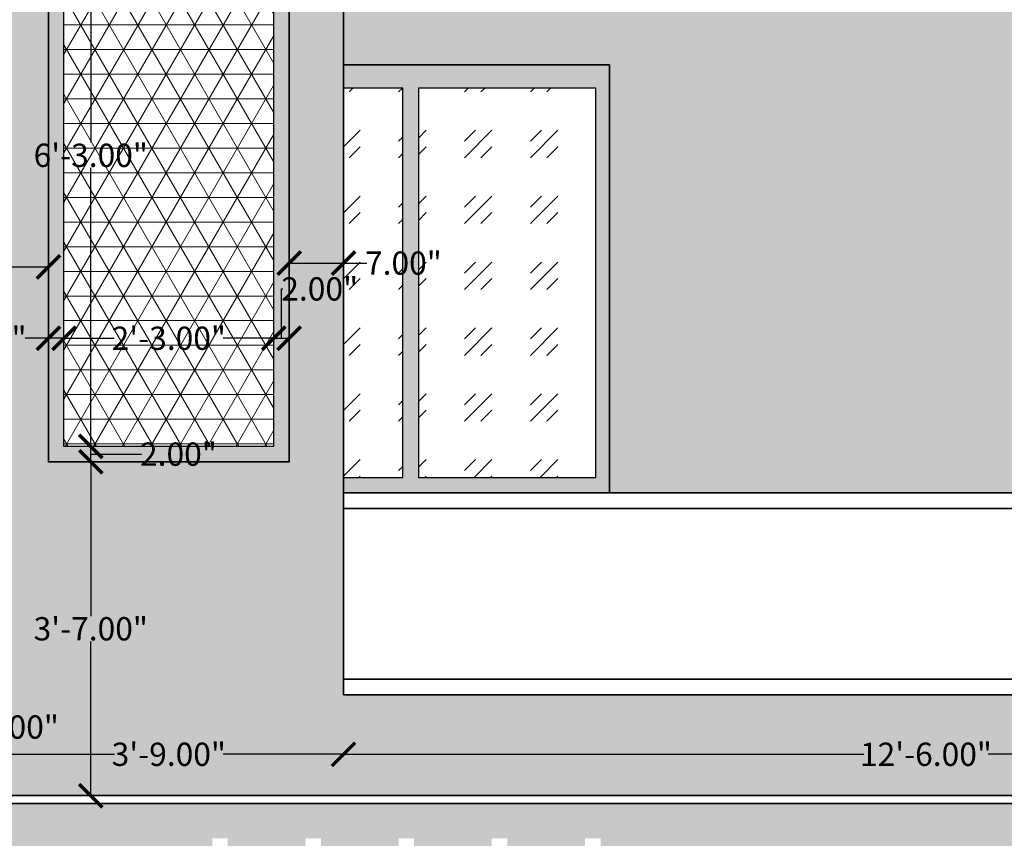
# Model space of a CAD drawing. Units: inches. Extents: x -654 to 390, y -40 to 648.
# Tile 7 of 13: x 104 to 231, y 311 to 417. Entities that reach past the tile are written whole.
import ezdxf

# ---------------------------------------------------------------- set-up
doc = ezdxf.new("R2010")
doc.units = ezdxf.units.IN
doc.header["$PDMODE"] = 3
for name, color, linetype, lineweight in [('A-ANNO-DIMS', 2, 'Continuous', 18), ('A-ELEV', 7, 'Continuous', 35), ('A-ELEV-FILL', 252, 'Continuous', 13), ('A-ELEV-PATT', 8, 'Continuous', 13), ('A-GLAZ', 4, 'Continuous', 25)]:
    doc.layers.add(name, color=color, linetype=linetype, lineweight=lineweight)
doc.styles.get("Standard").update_dxf_attribs({"font": 'arial.ttf'})
doc.dimstyles.get("Standard").update_dxf_attribs({"dimtxt": 3, "dimasz": 3, "dimexe": 0.18, "dimexo": 0.0625, "dimgap": 0.09, "dimtad": 0, "dimtih": 1, "dimtoh": 1, "dimzin": 0, "dimdsep": 46, "dimlunit": 3, "dimtxsty": 'Standard', "dimblk": 'ARCHTICK', "dimcen": 0.09, "dimse1": 1, "dimse2": 1, "dimadec": 0, "dimazin": 0, "dimtfac": 1, "dimtofl": 0, "dimtmove": 0, "dimatfit": 3, "dimfxl": 1, "dimtolj": 1, "dimtzin": 0, "dimarcsym": 0})

# ---------------------------------------------------------------- blocks, each defined once
blk = doc.blocks.new('_ArchTick')
at = {"color": 0, "linetype": 'ByBlock', "const_width": 0.15}
blk.add_lwpolyline([(-0.5, -0.5), (0.5, 0.5)], dxfattribs=at)
blk = doc.blocks.new('*D45')
at = {"layer": 'A-ANNO-DIMS', "color": 0, "lineweight": -2, "transparency": 16777216}
for p, q in [((99.15, 322.17), (99.15, 325.47)), ((99.15, 325.47), (99.33, 325.47)), ((100.65, 322.17), (97.65, 322.17))]:
    blk.add_line(p, q, dxfattribs=at)
at = {"layer": 'Defpoints', "color": 0, "transparency": 16777216}
for p in [(97.65, 322.17), (97.65, 316.63), (100.65, 316.63)]:
    blk.add_point(p, dxfattribs=at)
at = {"layer": 'A-ANNO-DIMS', "color": 0, "lineweight": -2, "transparency": 16777216, "xscale": 3, "yscale": 3, "zscale": 3, "rotation": 180}
blk.add_blockref('_ArchTick', (97.65, 322.17), dxfattribs=at)
at = {"layer": 'A-ANNO-DIMS', "color": 0, "lineweight": -2, "transparency": 16777216, "xscale": 3, "yscale": 3, "zscale": 3}
blk.add_blockref('_ArchTick', (100.65, 322.17), dxfattribs=at)
at = {"layer": 'A-ANNO-DIMS', "color": 0, "transparency": 16777216, "insert": (104.05, 325.47), "char_height": 3, "attachment_point": 5}
blk.add_mtext('\\A1;3.00"', dxfattribs=at)
blk = doc.blocks.new('*D46')
at = {"layer": 'A-ANNO-DIMS', "color": 0, "lineweight": -2, "transparency": 16777216}
for p, q in [((145.65, 321.96), (212.63, 321.96)), ((295.65, 321.96), (228.66, 321.96))]:
    blk.add_line(p, q, dxfattribs=at)
at = {"layer": 'Defpoints', "color": 0, "transparency": 16777216}
for p in [(145.65, 329.63), (145.65, 321.96), (295.65, 316.63)]:
    blk.add_point(p, dxfattribs=at)
at = {"layer": 'A-ANNO-DIMS', "color": 0, "lineweight": -2, "transparency": 16777216, "xscale": 3, "yscale": 3, "zscale": 3, "rotation": 180}
blk.add_blockref('_ArchTick', (145.65, 321.96), dxfattribs=at)
at = {"layer": 'A-ANNO-DIMS', "color": 0, "lineweight": -2, "transparency": 16777216, "xscale": 3, "yscale": 3, "zscale": 3}
blk.add_blockref('_ArchTick', (295.65, 321.96), dxfattribs=at)
at = {"layer": 'A-ANNO-DIMS', "color": 0, "transparency": 16777216, "insert": (220.65, 321.96), "char_height": 3, "attachment_point": 5}
blk.add_mtext('\\A1;12\'-6.00"', dxfattribs=at)
blk = doc.blocks.new('*D47')
at = {"layer": 'A-ANNO-DIMS', "color": 0, "lineweight": -2, "transparency": 16777216}
for p, q in [((100.65, 321.96), (116.16, 321.96)), ((145.65, 321.96), (130.14, 321.96))]:
    blk.add_line(p, q, dxfattribs=at)
at = {"layer": 'Defpoints', "color": 0, "transparency": 16777216}
for p in [(145.65, 329.63), (100.65, 322.17), (100.65, 321.96)]:
    blk.add_point(p, dxfattribs=at)
at = {"layer": 'A-ANNO-DIMS', "color": 0, "lineweight": -2, "transparency": 16777216, "xscale": 3, "yscale": 3, "zscale": 3, "rotation": 180}
blk.add_blockref('_ArchTick', (100.65, 321.96), dxfattribs=at)
at = {"layer": 'A-ANNO-DIMS', "color": 0, "lineweight": -2, "transparency": 16777216, "xscale": 3, "yscale": 3, "zscale": 3}
blk.add_blockref('_ArchTick', (145.65, 321.96), dxfattribs=at)
at = {"layer": 'A-ANNO-DIMS', "color": 0, "transparency": 16777216, "insert": (123.15, 321.96), "char_height": 3, "attachment_point": 5}
blk.add_mtext('\\A1;3\'-9.00"', dxfattribs=at)
blk = doc.blocks.new('*D48')
at = {"layer": 'A-ANNO-DIMS', "color": 0, "lineweight": -2, "transparency": 16777216}
for p, q in [((113.1, 359.63), (113.1, 339.76)), ((113.1, 316.63), (113.1, 336.51))]:
    blk.add_line(p, q, dxfattribs=at)
at = {"layer": 'Defpoints', "color": 0, "transparency": 16777216}
for p in [(107.65, 359.63), (113.1, 359.63), (100.65, 316.63)]:
    blk.add_point(p, dxfattribs=at)
at = {"layer": 'A-ANNO-DIMS', "color": 0, "lineweight": -2, "transparency": 16777216, "xscale": 3, "yscale": 3, "zscale": 3}
for p, rotation in [((113.1, 359.63), 90), ((113.1, 316.63), 270)]:
    blk.add_blockref('_ArchTick', p, dxfattribs=dict(at, rotation=rotation))
at = {"layer": 'A-ANNO-DIMS', "color": 0, "transparency": 16777216, "insert": (113.1, 338.13), "char_height": 3, "attachment_point": 5}
blk.add_mtext('\\A1;3\'-7.00"', dxfattribs=at)
blk = doc.blocks.new('*D49')
at = {"layer": 'A-ANNO-DIMS', "color": 0, "lineweight": -2, "transparency": 16777216}
for p, q in [((113.1, 359.63), (113.1, 361.63)), ((113.1, 360.63), (119.45, 360.63)), ((119.45, 360.63), (119.63, 360.63))]:
    blk.add_line(p, q, dxfattribs=at)
at = {"layer": 'Defpoints', "color": 0, "transparency": 16777216}
for p in [(113.1, 361.63), (113.1, 361.63), (107.65, 359.63)]:
    blk.add_point(p, dxfattribs=at)
at = {"layer": 'A-ANNO-DIMS', "color": 0, "lineweight": -2, "transparency": 16777216, "xscale": 3, "yscale": 3, "zscale": 3}
for p, rotation in [((113.1, 361.63), 90), ((113.1, 359.63), 270)]:
    blk.add_blockref('_ArchTick', p, dxfattribs=dict(at, rotation=rotation))
at = {"layer": 'A-ANNO-DIMS', "color": 0, "transparency": 16777216, "insert": (124.39, 360.63), "char_height": 3, "attachment_point": 5}
blk.add_mtext('\\A1;2.00"', dxfattribs=at)
blk = doc.blocks.new('*D50')
at = {"layer": 'A-ANNO-DIMS', "color": 0, "lineweight": -2, "transparency": 16777216}
for p, q in [((113.1, 436.63), (113.1, 400.76)), ((113.1, 361.63), (113.1, 397.51))]:
    blk.add_line(p, q, dxfattribs=at)
at = {"layer": 'Defpoints', "color": 0, "transparency": 16777216}
for p in [(113.1, 436.63), (113.1, 436.63), (113.1, 361.63)]:
    blk.add_point(p, dxfattribs=at)
at = {"layer": 'A-ANNO-DIMS', "color": 0, "lineweight": -2, "transparency": 16777216, "xscale": 3, "yscale": 3, "zscale": 3}
for p, rotation in [((113.1, 436.63), 90), ((113.1, 361.63), 270)]:
    blk.add_blockref('_ArchTick', p, dxfattribs=dict(at, rotation=rotation))
at = {"layer": 'A-ANNO-DIMS', "color": 0, "transparency": 16777216, "insert": (113.1, 399.13), "char_height": 3, "attachment_point": 5}
blk.add_mtext('\\A1;6\'-3.00"', dxfattribs=at)
blk = doc.blocks.new('*D53')
at = {"layer": 'A-ANNO-DIMS', "color": 0, "lineweight": -2, "transparency": 16777216}
for p, q in [((100.65, 384.74), (97.65, 384.74)), ((107.65, 384.74), (100.65, 384.74))]:
    blk.add_line(p, q, dxfattribs=at)
at = {"layer": 'Defpoints', "color": 0, "transparency": 16777216}
for p in [(100.65, 384.74), (100.65, 359.63), (107.65, 359.63)]:
    blk.add_point(p, dxfattribs=at)
at = {"layer": 'A-ANNO-DIMS', "color": 0, "lineweight": -2, "transparency": 16777216, "xscale": 3, "yscale": 3, "zscale": 3, "rotation": 180}
blk.add_blockref('_ArchTick', (100.65, 384.74), dxfattribs=at)
at = {"layer": 'A-ANNO-DIMS', "color": 0, "lineweight": -2, "transparency": 16777216, "xscale": 3, "yscale": 3, "zscale": 3}
blk.add_blockref('_ArchTick', (107.65, 384.74), dxfattribs=at)
at = {"layer": 'A-ANNO-DIMS', "color": 0, "transparency": 16777216, "insert": (92.93, 384.74), "char_height": 3, "attachment_point": 5}
blk.add_mtext('\\A1;7.00"', dxfattribs=at)
blk = doc.blocks.new('*D54')
at = {"layer": 'A-ANNO-DIMS', "color": 0, "lineweight": -2, "transparency": 16777216}
for p, q in [((107.65, 375.56), (104.65, 375.56)), ((109.65, 375.56), (107.65, 375.56))]:
    blk.add_line(p, q, dxfattribs=at)
at = {"layer": 'Defpoints', "color": 0, "transparency": 16777216}
for p in [(107.65, 375.56), (107.65, 361.63), (109.65, 361.63)]:
    blk.add_point(p, dxfattribs=at)
at = {"layer": 'A-ANNO-DIMS', "color": 0, "lineweight": -2, "transparency": 16777216, "xscale": 3, "yscale": 3, "zscale": 3, "rotation": 180}
blk.add_blockref('_ArchTick', (107.65, 375.56), dxfattribs=at)
at = {"layer": 'A-ANNO-DIMS', "color": 0, "lineweight": -2, "transparency": 16777216, "xscale": 3, "yscale": 3, "zscale": 3}
blk.add_blockref('_ArchTick', (109.65, 375.56), dxfattribs=at)
at = {"layer": 'A-ANNO-DIMS', "color": 0, "transparency": 16777216, "insert": (99.89, 375.56), "char_height": 3, "attachment_point": 5}
blk.add_mtext('\\A1;2.00"', dxfattribs=at)
blk = doc.blocks.new('*D55')
at = {"layer": 'A-ANNO-DIMS', "color": 0, "lineweight": -2, "transparency": 16777216}
for p, q in [((109.65, 375.56), (116.13, 375.56)), ((136.65, 375.56), (130.16, 375.56))]:
    blk.add_line(p, q, dxfattribs=at)
at = {"layer": 'Defpoints', "color": 0, "transparency": 16777216}
for p in [(109.65, 375.56), (136.65, 375.56), (136.65, 375.56)]:
    blk.add_point(p, dxfattribs=at)
at = {"layer": 'A-ANNO-DIMS', "color": 0, "lineweight": -2, "transparency": 16777216, "xscale": 3, "yscale": 3, "zscale": 3, "rotation": 180}
blk.add_blockref('_ArchTick', (109.65, 375.56), dxfattribs=at)
at = {"layer": 'A-ANNO-DIMS', "color": 0, "lineweight": -2, "transparency": 16777216, "xscale": 3, "yscale": 3, "zscale": 3}
blk.add_blockref('_ArchTick', (136.65, 375.56), dxfattribs=at)
at = {"layer": 'A-ANNO-DIMS', "color": 0, "transparency": 16777216, "insert": (123.15, 375.56), "char_height": 3, "attachment_point": 5}
blk.add_mtext('\\A1;2\'-3.00"', dxfattribs=at)
blk = doc.blocks.new('*D56')
at = {"layer": 'A-ANNO-DIMS', "color": 0, "lineweight": -2, "transparency": 16777216}
for p, q in [((137.65, 375.56), (137.65, 381.92)), ((137.65, 381.92), (137.83, 381.92)), ((136.65, 375.56), (138.65, 375.56))]:
    blk.add_line(p, q, dxfattribs=at)
at = {"layer": 'Defpoints', "color": 0, "transparency": 16777216}
for p in [(136.65, 375.56), (138.65, 375.56), (138.65, 375.56)]:
    blk.add_point(p, dxfattribs=at)
at = {"layer": 'A-ANNO-DIMS', "color": 0, "lineweight": -2, "transparency": 16777216, "xscale": 3, "yscale": 3, "zscale": 3, "rotation": 180}
blk.add_blockref('_ArchTick', (136.65, 375.56), dxfattribs=at)
at = {"layer": 'A-ANNO-DIMS', "color": 0, "lineweight": -2, "transparency": 16777216, "xscale": 3, "yscale": 3, "zscale": 3}
blk.add_blockref('_ArchTick', (138.65, 375.56), dxfattribs=at)
at = {"layer": 'A-ANNO-DIMS', "color": 0, "transparency": 16777216, "insert": (142.58, 381.92), "char_height": 3, "attachment_point": 5}
blk.add_mtext('\\A1;2.00"', dxfattribs=at)
blk = doc.blocks.new('*D57')
at = {"layer": 'A-ANNO-DIMS', "color": 0, "lineweight": -2, "transparency": 16777216}
for p, q in [((138.65, 385.24), (145.65, 385.24)), ((145.65, 385.24), (148.65, 385.24))]:
    blk.add_line(p, q, dxfattribs=at)
at = {"layer": 'Defpoints', "color": 0, "transparency": 16777216}
for p in [(145.65, 385.24), (138.65, 359.63), (145.65, 359.63)]:
    blk.add_point(p, dxfattribs=at)
at = {"layer": 'A-ANNO-DIMS', "color": 0, "lineweight": -2, "transparency": 16777216, "xscale": 3, "yscale": 3, "zscale": 3, "rotation": 180}
blk.add_blockref('_ArchTick', (138.65, 385.24), dxfattribs=at)
at = {"layer": 'A-ANNO-DIMS', "color": 0, "lineweight": -2, "transparency": 16777216, "xscale": 3, "yscale": 3, "zscale": 3}
blk.add_blockref('_ArchTick', (145.65, 385.24), dxfattribs=at)
at = {"layer": 'A-ANNO-DIMS', "color": 0, "transparency": 16777216, "insert": (153.36, 385.24), "char_height": 3, "attachment_point": 5}
blk.add_mtext('\\A1;7.00"', dxfattribs=at)
blk = doc.blocks.new('*D76')
at = {"layer": 'A-ANNO-DIMS', "color": 0, "lineweight": -2, "transparency": 16777216}
for p, q in [((380.75, 611.13), (380.75, 306.76)), ((380.75, -0.87), (380.75, 303.51))]:
    blk.add_line(p, q, dxfattribs=at)
at = {"layer": 'Defpoints', "color": 0, "transparency": 16777216}
for p in [(126.65, 611.13), (380.75, 611.13), (346.65, -0.87)]:
    blk.add_point(p, dxfattribs=at)
at = {"layer": 'A-ANNO-DIMS', "color": 0, "lineweight": -2, "transparency": 16777216, "xscale": 3, "yscale": 3, "zscale": 3}
for p, rotation in [((380.75, 611.13), 90), ((380.75, -0.87), 270)]:
    blk.add_blockref('_ArchTick', p, dxfattribs=dict(at, rotation=rotation))
at = {"layer": 'A-ANNO-DIMS', "color": 0, "transparency": 16777216, "insert": (380.75, 305.13), "char_height": 3, "attachment_point": 5}
blk.add_mtext('\\A1;51\'-0"', dxfattribs=at)
blk = doc.blocks.new('*D96')
at = {"layer": 'A-ANNO-DIMS', "color": 0, "lineweight": -2, "transparency": 16777216}
for p, q in [((128.74, 643.23), (130.74, 643.23)), ((130.74, 643.23), (133.74, 643.23))]:
    blk.add_line(p, q, dxfattribs=at)
at = {"layer": 'Defpoints', "color": 0, "transparency": 16777216}
for p in [(130.74, 643.23), (128.74, 311.13), (130.74, 311.13)]:
    blk.add_point(p, dxfattribs=at)
at = {"layer": 'A-ANNO-DIMS', "color": 0, "lineweight": -2, "transparency": 16777216, "xscale": 3, "yscale": 3, "zscale": 3, "rotation": 180}
blk.add_blockref('_ArchTick', (128.74, 643.23), dxfattribs=at)
at = {"layer": 'A-ANNO-DIMS', "color": 0, "lineweight": -2, "transparency": 16777216, "xscale": 3, "yscale": 3, "zscale": 3}
blk.add_blockref('_ArchTick', (130.74, 643.23), dxfattribs=at)
at = {"layer": 'A-ANNO-DIMS', "color": 0, "transparency": 16777216, "insert": (137.82, 643.23), "char_height": 3, "attachment_point": 5}
blk.add_mtext('\\A1;0\'-2"', dxfattribs=at)
blk = doc.blocks.new('*D99')
at = {"layer": 'A-ANNO-DIMS', "color": 0, "lineweight": -2, "transparency": 16777216}
for p, q in [((380.75, 311.13), (380.75, 243.76)), ((380.75, 173.13), (380.75, 240.51))]:
    blk.add_line(p, q, dxfattribs=at)
at = {"layer": 'Defpoints', "color": 0, "transparency": 16777216}
for p in [(178.74, 311.13), (380.75, 311.13), (178.74, 173.13)]:
    blk.add_point(p, dxfattribs=at)
at = {"layer": 'A-ANNO-DIMS', "color": 0, "lineweight": -2, "transparency": 16777216, "xscale": 3, "yscale": 3, "zscale": 3}
for p, rotation in [((380.75, 311.13), 90), ((380.75, 173.13), 270)]:
    blk.add_blockref('_ArchTick', p, dxfattribs=dict(at, rotation=rotation))
at = {"layer": 'A-ANNO-DIMS', "color": 0, "transparency": 16777216, "insert": (380.75, 242.13), "char_height": 3, "attachment_point": 5}
blk.add_mtext('\\A1;11\'-6"', dxfattribs=at)
blk = doc.blocks.new('*D100')
at = {"layer": 'A-ANNO-DIMS', "color": 0, "lineweight": -2, "transparency": 16777216}
for p, q in [((145.65, -32.97), (157.49, -32.97)), ((179.88, -32.97), (168.03, -32.97))]:
    blk.add_line(p, q, dxfattribs=at)
at = {"layer": 'Defpoints', "color": 0, "transparency": 16777216}
for p in [(145.65, 355.63), (179.88, 355.63), (179.88, -32.97)]:
    blk.add_point(p, dxfattribs=at)
at = {"layer": 'A-ANNO-DIMS', "color": 0, "lineweight": -2, "transparency": 16777216, "xscale": 3, "yscale": 3, "zscale": 3, "rotation": 180}
blk.add_blockref('_ArchTick', (145.65, -32.97), dxfattribs=at)
at = {"layer": 'A-ANNO-DIMS', "color": 0, "lineweight": -2, "transparency": 16777216, "xscale": 3, "yscale": 3, "zscale": 3}
blk.add_blockref('_ArchTick', (179.88, -32.97), dxfattribs=at)
at = {"layer": 'A-ANNO-DIMS', "color": 0, "transparency": 16777216, "insert": (162.76, -32.97), "char_height": 3, "attachment_point": 5}
blk.add_mtext('\\A1;2\'-10"', dxfattribs=at)
blk = doc.blocks.new('*D101')
at = {"layer": 'A-ANNO-DIMS', "color": 0, "lineweight": -2, "transparency": 16777216}
for p, q in [((-35.45, 410.79), (-35.45, 384.8)), ((-35.45, 355.63), (-35.45, 381.62))]:
    blk.add_line(p, q, dxfattribs=at)
at = {"layer": 'Defpoints', "color": 0, "transparency": 16777216}
for p in [(-35.45, 410.79), (239.87, 410.79), (239.87, 355.63)]:
    blk.add_point(p, dxfattribs=at)
at = {"layer": 'A-ANNO-DIMS', "color": 0, "lineweight": -2, "transparency": 16777216, "xscale": 3, "yscale": 3, "zscale": 3}
for p, rotation in [((-35.45, 410.79), 90), ((-35.45, 355.63), 270)]:
    blk.add_blockref('_ArchTick', p, dxfattribs=dict(at, rotation=rotation))
at = {"layer": 'A-ANNO-DIMS', "color": 0, "transparency": 16777216, "insert": (-35.45, 383.21), "char_height": 3, "attachment_point": 5}
blk.add_mtext('\\A1;4\'-7"', dxfattribs=at)
blk = doc.blocks.new('*D102')
at = {"layer": 'A-ANNO-DIMS', "color": 0, "lineweight": -2, "transparency": 16777216}
for p, q in [((179.88, -32.97), (205.8, -32.97)), ((239.87, -32.97), (213.95, -32.97))]:
    blk.add_line(p, q, dxfattribs=at)
at = {"layer": 'Defpoints', "color": 0, "transparency": 16777216}
for p in [(179.88, 355.63), (239.87, 355.63), (239.87, -32.97)]:
    blk.add_point(p, dxfattribs=at)
at = {"layer": 'A-ANNO-DIMS', "color": 0, "lineweight": -2, "transparency": 16777216, "xscale": 3, "yscale": 3, "zscale": 3, "rotation": 180}
blk.add_blockref('_ArchTick', (179.88, -32.97), dxfattribs=at)
at = {"layer": 'A-ANNO-DIMS', "color": 0, "lineweight": -2, "transparency": 16777216, "xscale": 3, "yscale": 3, "zscale": 3}
blk.add_blockref('_ArchTick', (239.87, -32.97), dxfattribs=at)
at = {"layer": 'A-ANNO-DIMS', "color": 0, "transparency": 16777216, "insert": (209.87, -32.97), "char_height": 3, "attachment_point": 5}
blk.add_mtext('\\A1;5\'-0"', dxfattribs=at)

msp = doc.modelspace()

# ---------------------------------------------------------------- hatches: boundary and pattern name
at = {"layer": 'A-ELEV-FILL'}
h = msp.add_hatch(color=256, dxfattribs=at)
h.dxf.hatch_style = 1
h.paths.add_polyline_path([(346.646, 587.634), (161.035, 587.634), (161.035, 583.634), (342.646, 583.634), (342.646, 497.134), (346.646, 497.134), (346.646, 583.634)])
h.paths.add_polyline_path([(295.646, 315.634), (98.293, 315.634), (98.293, 311.134), (295.646, 311.134)])
h.paths.add_polyline_path([(128.742, 311.134), (98.293, 311.134), (98.293, 306.634), (128.742, 306.634)])
h.paths.add_polyline_path([(140.742, 311.134), (130.742, 311.134), (130.742, 306.634), (140.742, 306.634)])
h.paths.add_polyline_path([(152.742, 311.134), (142.742, 311.134), (142.742, 306.634), (152.742, 306.634)])
h.paths.add_polyline_path([(164.742, 311.134), (154.742, 311.134), (154.742, 306.634), (164.742, 306.634)])
h.paths.add_polyline_path([(176.742, 311.134), (166.742, 311.134), (166.742, 306.634), (176.742, 306.634)])
h.paths.add_polyline_path([(295.646, 311.134), (178.742, 311.134), (178.742, 306.634), (295.646, 306.634)])
h.paths.add_polyline_path([(303.818, 315.634), (295.646, 315.634), (295.646, 311.134), (303.818, 311.134)])
h.paths.add_polyline_path([(303.818, 311.134), (295.646, 311.134), (295.646, 306.634), (303.818, 306.634)])
h = msp.add_hatch(color=256, dxfattribs=at)
h.dxf.hatch_style = 1
h.paths.add_polyline_path([(295.646, 190.634), (178.742, 190.634), (178.742, 177.634), (295.646, 177.634)])
h.paths.add_polyline_path([(176.742, 190.634), (166.742, 190.634), (166.742, 177.634), (176.742, 177.634)])
h.paths.add_polyline_path([(164.742, 190.634), (154.742, 190.634), (154.742, 177.634), (164.742, 177.634)])
h.paths.add_polyline_path([(152.742, 190.634), (142.742, 190.634), (142.742, 177.634), (152.742, 177.634)])
h.paths.add_polyline_path([(140.742, 190.634), (130.742, 190.634), (130.742, 177.634), (140.742, 177.634)])
h.paths.add_polyline_path([(128.742, 190.634), (120.146, 190.634), (120.146, 177.634), (128.742, 177.634)])
h.paths.add_polyline_path([(295.646, 329.634), (145.646, 329.634), (145.646, 442.634), (100.646, 442.634), (100.646, 316.634), (295.646, 316.634)])
h.paths.add_polyline_path([(138.646, 359.634), (107.646, 359.634), (107.646, 438.634), (138.646, 438.634)], flags=16)
h.paths.add_polyline_path([(136.646, 361.634), (109.646, 361.634), (109.646, 436.634), (136.646, 436.634)], flags=0)
h.paths.add_polyline_path([(184.646, 466.634), (7.646, 466.634), (7.646, 453.634), (184.646, 453.634)])
h.paths.add_polyline_path([(184.646, 494.634), (7.646, 494.634), (7.646, 492.634), (184.646, 492.634)])
h.paths.add_polyline_path([(10.336, 492.634), (9.336, 492.634), (9.336, 468.634), (10.336, 468.634)])
h.paths.add_polyline_path([(17.352, 492.634), (16.352, 492.634), (16.352, 468.634), (17.352, 468.634)])
h.paths.add_polyline_path([(24.368, 492.634), (23.368, 492.634), (23.368, 468.634), (24.368, 468.634)])
h.paths.add_polyline_path([(31.384, 492.634), (30.384, 492.634), (30.384, 468.634), (31.384, 468.634)])
h.paths.add_polyline_path([(38.4, 492.634), (37.4, 492.634), (37.4, 468.634), (38.4, 468.634)])
h.paths.add_polyline_path([(45.416, 492.634), (44.416, 492.634), (44.416, 468.634), (45.416, 468.634)])
h.paths.add_polyline_path([(52.432, 492.634), (51.432, 492.634), (51.432, 468.634), (52.432, 468.634)])
h.paths.add_polyline_path([(59.448, 492.634), (58.448, 492.634), (58.448, 468.634), (59.448, 468.634)])
h.paths.add_polyline_path([(66.464, 492.634), (65.464, 492.634), (65.464, 468.634), (66.464, 468.634)])
h.paths.add_polyline_path([(73.48, 492.634), (72.48, 492.634), (72.48, 468.634), (73.48, 468.634)])
h.paths.add_polyline_path([(80.496, 492.634), (79.496, 492.634), (79.496, 468.634), (80.496, 468.634)])
h.paths.add_polyline_path([(87.512, 492.634), (86.512, 492.634), (86.512, 468.634), (87.512, 468.634)])
h.paths.add_polyline_path([(94.528, 492.634), (93.528, 492.634), (93.528, 468.634), (94.528, 468.634)])
h.paths.add_polyline_path([(101.544, 492.634), (100.544, 492.634), (100.544, 468.634), (101.544, 468.634)])
h.paths.add_polyline_path([(108.559, 492.634), (107.559, 492.634), (107.559, 468.634), (108.559, 468.634)])
h.paths.add_polyline_path([(115.575, 492.634), (114.575, 492.634), (114.575, 468.634), (115.575, 468.634)])
h.paths.add_polyline_path([(122.591, 492.634), (121.591, 492.634), (121.591, 468.634), (122.591, 468.634)])
h.paths.add_polyline_path([(129.607, 492.634), (128.607, 492.634), (128.607, 468.634), (129.607, 468.634)])
h.paths.add_polyline_path([(136.623, 492.634), (135.623, 492.634), (135.623, 468.634), (136.623, 468.634)])
h.paths.add_polyline_path([(143.639, 492.634), (142.639, 492.634), (142.639, 468.634), (143.639, 468.634)])
h.paths.add_polyline_path([(150.655, 492.634), (149.655, 492.634), (149.655, 468.634), (150.655, 468.634)])
h.paths.add_polyline_path([(157.671, 492.634), (156.671, 492.634), (156.671, 468.634), (157.671, 468.634)])
h.paths.add_polyline_path([(164.687, 492.634), (163.687, 492.634), (163.687, 468.634), (164.687, 468.634)])
h.paths.add_polyline_path([(171.703, 492.634), (170.703, 492.634), (170.703, 468.634), (171.703, 468.634)])
h.paths.add_polyline_path([(178.719, 492.634), (177.719, 492.634), (177.719, 468.634), (178.719, 468.634)])
h = msp.add_hatch(color=256, dxfattribs=at)
h.dxf.hatch_style = 1
h.paths.add_polyline_path([(239.871, 410.786), (291.141, 410.786), (291.141, 355.634), (295.646, 355.634), (295.646, 442.634), (145.646, 442.634), (145.646, 410.786), (179.877, 410.786), (179.877, 355.634), (239.871, 355.634)])
h = msp.add_hatch(color=256, dxfattribs=at)
h.dxf.hatch_style = 1
h.paths.add_polyline_path([(138.646, 438.634), (107.646, 438.634), (107.646, 359.634), (138.646, 359.634)])
h.paths.add_polyline_path([(136.646, 436.634), (136.646, 361.634), (109.646, 361.634), (109.646, 436.634)], flags=16)
h.paths.add_polyline_path([(179.877, 410.786), (145.646, 410.786), (145.646, 407.786), (153.285, 407.786), (153.285, 357.634), (145.646, 357.634), (145.646, 355.634), (179.877, 355.634)])
h.paths.add_polyline_path([(178.123, 407.786), (178.123, 357.634), (155.286, 357.634), (155.286, 407.786)], flags=16)
h.paths.add_polyline_path([(291.141, 410.786), (239.871, 410.786), (239.871, 355.634), (241.996, 355.634), (241.996, 407.786), (269.317, 407.786), (269.317, 355.634), (271.318, 355.634), (271.318, 407.786), (289.369, 407.786), (289.369, 355.634), (291.141, 355.634)])
h.paths.add_polyline_path([(128.225, 268.786), (128.742, 268.786), (128.742, 271.786), (125.225, 271.786), (125.225, 216.634), (128.225, 216.634)])
h.paths.add_polyline_path([(140.742, 271.786), (130.742, 271.786), (130.742, 268.786), (140.742, 268.786)])
h.paths.add_polyline_path([(152.742, 271.786), (142.742, 271.786), (142.742, 268.786), (152.742, 268.786)])
h.paths.add_polyline_path([(164.742, 271.786), (154.742, 271.786), (154.742, 268.786), (164.742, 268.786)])
h.paths.add_polyline_path([(176.742, 271.786), (167.328, 271.786), (166.742, 271.786), (166.742, 268.786), (167.328, 268.786), (167.328, 216.634), (169.328, 216.634), (169.328, 268.786), (176.742, 268.786)])
h.paths.add_polyline_path([(221.328, 271.786), (178.742, 271.786), (178.742, 268.786), (184.828, 268.786), (184.828, 216.634), (186.829, 216.634), (186.829, 268.786), (202.329, 268.786), (202.329, 216.634), (204.325, 216.634), (204.325, 268.786), (219.825, 268.786), (219.825, 216.634), (221.328, 216.634)])
h.paths.add_polyline_path([(295.646, 271.786), (244.726, 271.786), (244.726, 216.634), (246.481, 216.634), (246.481, 268.786), (269.317, 268.786), (269.317, 216.634), (271.318, 216.634), (271.318, 268.786), (286.818, 268.786), (286.818, 216.634), (288.814, 216.634), (288.814, 268.786), (295.646, 268.786)])
h.paths.add_polyline_path([(295.646, 216.634), (178.742, 216.634), (178.742, 214.634), (295.646, 214.634)])
h.paths.add_polyline_path([(128.742, 216.634), (123.485, 216.634), (123.485, 214.634), (128.742, 214.634)])
h.paths.add_polyline_path([(140.742, 216.634), (130.742, 216.634), (130.742, 214.634), (140.742, 214.634)])
h.paths.add_polyline_path([(152.742, 216.634), (142.742, 216.634), (142.742, 214.634), (152.742, 214.634)])
h.paths.add_polyline_path([(164.742, 216.634), (154.742, 216.634), (154.742, 214.634), (164.742, 214.634)])
h.paths.add_polyline_path([(176.742, 216.634), (166.742, 216.634), (166.742, 214.634), (176.742, 214.634)])
h.paths.add_polyline_path([(128.742, 192.634), (119.386, 192.634), (119.386, 190.634), (128.742, 190.634)])
h.paths.add_polyline_path([(140.742, 192.634), (130.742, 192.634), (130.742, 190.634), (140.742, 190.634)])
h.paths.add_polyline_path([(152.742, 192.634), (142.742, 192.634), (142.742, 190.634), (152.742, 190.634)])
h.paths.add_polyline_path([(164.742, 192.634), (154.742, 192.634), (154.742, 190.634), (164.742, 190.634)])
h.paths.add_polyline_path([(176.742, 192.634), (166.742, 192.634), (166.742, 190.634), (176.742, 190.634)])
h.paths.add_polyline_path([(295.646, 192.634), (178.742, 192.634), (178.742, 190.634), (295.646, 190.634)])
h.paths.add_polyline_path([(189.362, 137.63), (135.362, 137.63), (135.362, 71.63), (189.362, 71.63)])
h.paths.add_polyline_path([(154.862, 134.63), (170.362, 134.63), (170.362, 74.63), (154.862, 74.63)], flags=16)
h.paths.add_polyline_path([(152.862, 134.63), (152.862, 74.63), (137.362, 74.63), (137.362, 134.63)], flags=16)
h.paths.add_polyline_path([(172.358, 134.63), (187.858, 134.63), (187.858, 74.63), (172.358, 74.63)], flags=16)
h.paths.add_polyline_path([(113.646, 83.134), (62.646, 83.134), (62.646, 17.134), (113.646, 17.134)])
h.paths.add_polyline_path([(96.484, 80.08), (109.984, 80.08), (109.984, 20.08), (96.484, 20.08)], flags=16)
h.paths.add_polyline_path([(93.843, 80.08), (93.843, 20.08), (80.343, 20.08), (80.343, 80.08)], flags=16)
h.paths.add_polyline_path([(78.051, 80.08), (78.051, 20.08), (64.551, 20.08), (64.551, 80.08)], flags=16)
h.paths.add_polyline_path([(60.646, 83.134), (9.646, 83.134), (9.646, 17.134), (60.646, 17.134)])
h.paths.add_polyline_path([(58.197, 80.08), (58.197, 20.08), (44.697, 20.08), (44.697, 80.08)], flags=16)
h.paths.add_polyline_path([(41.55, 80.08), (41.55, 20.08), (28.05, 20.08), (28.05, 80.08)], flags=16)
h.paths.add_polyline_path([(25.146, 80.08), (25.146, 20.08), (11.646, 20.08), (11.646, 80.08)], flags=16)
h.paths.add_polyline_path([(9.646, 83.134), (7.646, 83.134), (7.646, 73.776), (9.646, 73.776)])
h.paths.add_polyline_path([(9.646, 65.663), (7.646, 65.663), (7.646, 36.041), (9.646, 36.041)])
h.paths.add_polyline_path([(9.646, 27.928), (7.646, 27.928), (7.646, 17.134), (9.646, 17.134)])
h.paths.add_polyline_path([(115.646, 83.134), (113.646, 83.134), (113.646, 73.776), (115.646, 73.776)])
h.paths.add_polyline_path([(115.646, 65.663), (113.646, 65.663), (113.646, 35.502), (115.646, 35.502)])
h.paths.add_polyline_path([(115.646, 27.389), (113.646, 27.389), (113.646, 17.134), (115.646, 17.134)])
h.paths.add_polyline_path([(8.146, 89.642), (-1.854, 89.642), (-1.854, 87.642), (8.146, 87.642)])
h.paths.add_polyline_path([(245.646, 156.634), (243.646, 156.634), (243.646, 17.134), (245.646, 17.134)])
h.paths.add_polyline_path([(339.646, 156.634), (337.646, 156.634), (337.646, 17.134), (339.646, 17.134)])
at = {"layer": 'A-ELEV-PATT'}
h = msp.add_hatch(dxfattribs=at)
h.set_pattern_fill('NET3', color=256)
h.paths.add_polyline_path([(136.646, 436.634), (109.646, 436.634), (109.646, 361.634), (136.646, 361.634)])
h = msp.add_hatch(dxfattribs=at)
h.set_pattern_fill('GOST_GLASS', color=256)
h.paths.add_polyline_path([(289.369, 407.786), (271.318, 407.786), (271.318, 355.634), (289.369, 355.634)])
h.paths.add_polyline_path([(178.123, 407.786), (155.286, 407.786), (155.286, 357.634), (178.123, 357.634)])
h.paths.add_polyline_path([(153.285, 407.786), (145.646, 407.786), (145.646, 357.634), (153.285, 357.634)])
h.paths.add_polyline_path([(184.828, 268.786), (178.742, 268.786), (178.742, 216.634), (184.828, 216.634)])
h.paths.add_polyline_path([(176.742, 268.786), (169.328, 268.786), (169.328, 216.634), (176.742, 216.634)])
h.paths.add_polyline_path([(202.329, 268.786), (186.829, 268.786), (186.829, 216.634), (202.329, 216.634)])
h.paths.add_polyline_path([(219.825, 268.786), (204.325, 268.786), (204.325, 216.634), (219.825, 216.634)])
h.paths.add_polyline_path([(286.818, 268.786), (271.318, 268.786), (271.318, 216.634), (286.818, 216.634)])
h.paths.add_polyline_path([(295.646, 268.786), (288.814, 268.786), (288.814, 216.634), (295.646, 216.634)])

# ---------------------------------------------------------------- linework, layer by layer
at = {"layer": 'A-ELEV'}
for p, q in [((145.646, 329.634), (145.646, 442.634)), ((145.646, 355.634), (295.646, 355.634)), ((145.646, 353.634), (295.646, 353.634)), ((145.646, 331.634), (295.646, 331.634)), ((145.646, 329.634), (295.646, 329.634)), ((97.646, 316.634), (304.646, 316.634)), ((97.646, 315.634), (304.646, 315.634))]:
    msp.add_line(p, q, dxfattribs=at)
msp.add_lwpolyline([(107.646, 438.634), (138.646, 438.634), (138.646, 359.634), (107.646, 359.634)], close=True, dxfattribs=at)
msp.add_lwpolyline([(179.877, 355.634), (179.877, 410.786), (145.646, 410.786)], dxfattribs=at)
at = {"layer": 'A-GLAZ'}
for p, q in [((145.646, 357.634), (153.285, 357.634)), ((155.286, 357.634), (178.123, 357.634))]:
    msp.add_line(p, q, dxfattribs=at)
msp.add_lwpolyline([(109.646, 436.634), (136.646, 436.634), (136.646, 361.634), (109.646, 361.634)], close=True, dxfattribs=at)
for points in [[(153.285, 357.634), (153.285, 407.786), (145.646, 407.786)], [(178.123, 357.634), (178.123, 407.786), (155.286, 407.786), (155.286, 357.634)]]:
    msp.add_lwpolyline(points, dxfattribs=at)

# ---------------------------------------------------------------- dimensions: what is measured, and where the dimension line sits
at = {"layer": 'A-ANNO-DIMS'}
for base, p1, p2, override, picture, middle in [((130.742, 643.234), (128.742, 311.134), (130.742, 311.134), {"dimdec": 1, "dimlfac": 1, "dimrnd": 0, "dimzin": 1, "dimdsep": 46, "dimlunit": 4, "dimfrac": 2}, '*D96', (137.82, 643.234)), ((100.646, 384.745), (107.646, 359.634), (100.646, 359.634), {"dimclrd": 0, "dimclre": 0, "dimclrt": 0}, '*D53', (92.932, 384.745)), ((145.646, 385.239), (138.646, 359.634), (145.646, 359.634), {"dimclrd": 0, "dimclre": 0, "dimclrt": 0}, '*D57', (153.361, 385.239)), ((138.646, 375.564), (136.646, 375.564), (138.646, 375.564), {"dimclrd": 0, "dimclre": 0, "dimclrt": 0, "dimtmove": 1}, '*D56', (137.916, 381.916)), ((107.646, 375.564), (109.646, 361.634), (107.646, 361.634), {"dimclrd": 0, "dimclre": 0, "dimclrt": 0}, '*D54', (99.894, 375.564)), ((136.646, 375.564), (109.646, 375.564), (136.646, 375.564), {"dimclrd": 0, "dimclre": 0, "dimclrt": 0}, '*D55', (123.146, 375.564)), ((179.877, -32.966), (145.646, 355.634), (179.877, 355.634), {"dimdec": 1, "dimlfac": 1, "dimrnd": 0, "dimzin": 1, "dimdsep": 46, "dimlunit": 4, "dimfrac": 2}, '*D100', (162.762, -32.966)), ((239.871, -32.966), (179.877, 355.634), (239.871, 355.634), {"dimdec": 1, "dimlfac": 1, "dimrnd": 0, "dimzin": 1, "dimdsep": 46, "dimlunit": 4, "dimfrac": 2}, '*D102', (209.874, -32.966)), ((100.646, 321.96), (145.646, 329.634), (100.646, 322.175), {"dimclrd": 0, "dimclre": 0, "dimclrt": 0, "dimtmove": 1}, '*D47', (123.146, 321.96)), ((145.646, 321.96), (295.646, 316.634), (145.646, 329.634), {"dimclrd": 0, "dimclre": 0, "dimclrt": 0}, '*D46', (220.646, 321.96)), ((97.646, 322.175), (100.646, 316.634), (97.646, 316.634), {"dimclrd": 0, "dimclre": 0, "dimclrt": 0, "dimtmove": 1}, '*D45', (99.416, 325.465))]:
    dim = msp.add_linear_dim(base=base, p1=p1, p2=p2, dimstyle='Standard', override=override, dxfattribs=at)
    dim.commit()
    dim.dimension.update_dxf_attribs({"geometry": picture, "text_midpoint": middle})
for base, p1, p2, override, picture, middle in [((380.746, 611.134), (346.646, -0.866), (126.646, 611.134), {"dimdec": 1, "dimlfac": 1, "dimrnd": 0, "dimzin": 1, "dimdsep": 46, "dimlunit": 4, "dimfrac": 2}, '*D76', (380.746, 305.134)), ((113.102, 436.634), (113.102, 361.634), (113.102, 436.634), {"dimclrd": 0, "dimclre": 0, "dimclrt": 0, "dimtmove": 1}, '*D50', (113.102, 399.134)), ((-35.454, 410.786), (239.871, 355.634), (239.871, 410.786), {"dimdec": 1, "dimlfac": 1, "dimrnd": 0, "dimzin": 1, "dimdsep": 46, "dimlunit": 4, "dimfrac": 2}, '*D101', (-35.454, 383.21)), ((113.102, 361.634), (107.646, 359.634), (113.102, 361.634), {"dimclrd": 0, "dimclre": 0, "dimclrt": 0, "dimtmove": 1}, '*D49', (119.724, 360.634)), ((113.102, 359.634), (100.646, 316.634), (107.646, 359.634), {"dimclrd": 0, "dimclre": 0, "dimclrt": 0}, '*D48', (113.102, 338.134)), ((380.746, 311.134), (178.742, 173.134), (178.742, 311.134), {"dimdec": 1, "dimlfac": 1, "dimrnd": 0, "dimzin": 1, "dimdsep": 46, "dimlunit": 4, "dimfrac": 2}, '*D99', (380.746, 242.134))]:
    dim = msp.add_linear_dim(base=base, p1=p1, p2=p2, angle=90, dimstyle='Standard', override=override, dxfattribs=at)
    dim.commit()
    dim.dimension.update_dxf_attribs({"geometry": picture, "text_midpoint": middle})

doc.saveas('drawing.dxf')
